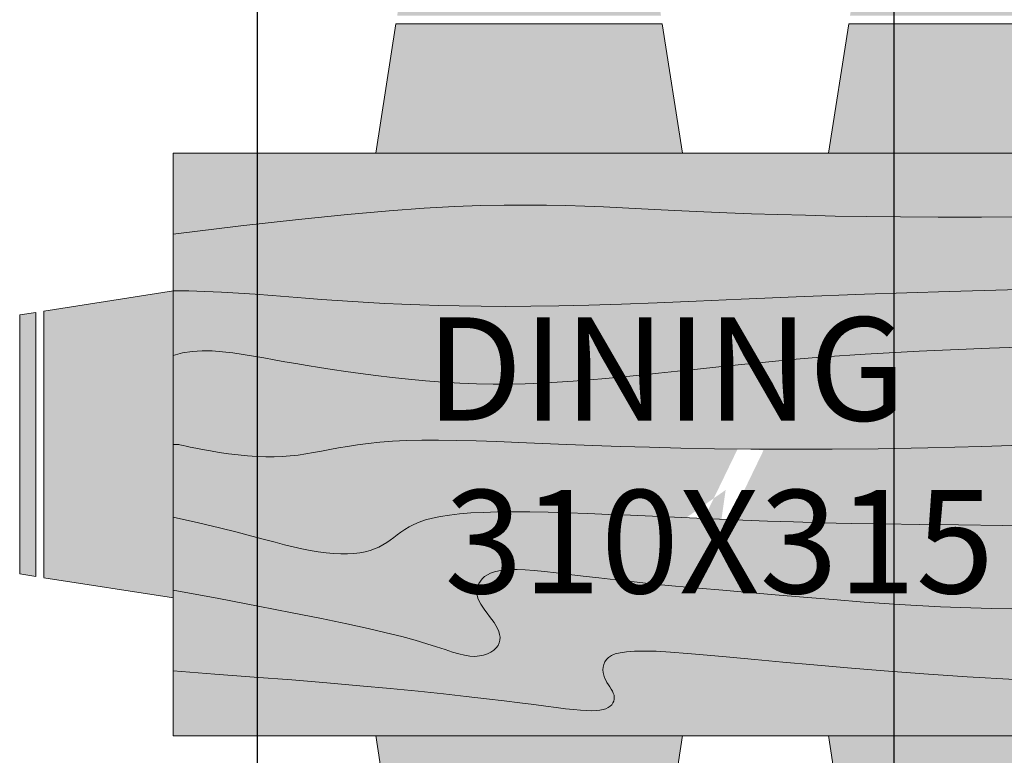
# Model space of a CAD drawing. Units: inches. Extents: x 192 to 1361, y -1362 to 367.
# Tile 16 of 23: x 498 to 662, y -337 to -214. Entities that reach past the tile are written whole.
import ezdxf

# ---------------------------------------------------------------- set-up
doc = ezdxf.new("R2010")
doc.units = ezdxf.units.IN
doc.header["$MEASUREMENT"] = 0
for name, color, linetype, lineweight in [('A-ANNO-DIMS', 2, 'Continuous', 18), ('A-AREA-IDEN', 7, 'Continuous', 18), ('furniture', 32, 'Continuous', 18)]:
    doc.layers.add(name, color=color, linetype=linetype, lineweight=lineweight)
doc.layers.add('A-FURN-PATT', color=254, linetype='Continuous', lineweight=13, true_color=0xfeeab9)
doc.styles.get("Standard").update_dxf_attribs({"font": 'arial.ttf'})
doc.dimstyles.get("Standard").update_dxf_attribs({"dimtxt": 0.18, "dimasz": 0.18, "dimexe": 0.18, "dimexo": 0.0625, "dimgap": 0.09, "dimtad": 0, "dimtih": 1, "dimtoh": 1, "dimzin": 0, "dimdsep": 46, "dimlunit": 3, "dimtxsty": 'Standard', "dimcen": 0.09, "dimadec": 0, "dimazin": 0, "dimtfac": 1, "dimtofl": 0, "dimtmove": 0, "dimatfit": 3, "dimfxl": 1, "dimtolj": 1, "dimtzin": 0, "dimarcsym": 0})

# ---------------------------------------------------------------- blocks, each defined once
blk = doc.blocks.new('Dining Set - 36 x 72 in.')
for p, q in [((-4.5152, 17.99762), (-5.7655, 25.99926)), ((5.7657, 26.00059), (4.5153, 17.99762)), ((23.4848, 17.99762), (22.2345, 25.99926)), ((36, 18), (-36, 18)), ((36, -18), (36, 18)), ((44.0006, 8.23428), (35.9976, 9.48474)), ((44, 8.23041), (44, -8.23915)), ((44.5, -8.15843), (44.5, 8.15338)), ((45.5, 8), (44.5005, 8.15617)), ((45.5, 8), (45.5, -8)), ((35.9976, -9.48476), (43.9993, -8.2345)), ((44.4997, -8.15631), (45.5, -8)), ((-36, -18), (36, -18)), ((-4.5152, -17.99762), (-5.7655, -25.99928)), ((5.7657, -26.0006), (4.5153, -17.99762)), ((23.4848, -17.99762), (22.2345, -25.99928)), ((-22.2304, -26), (-5.7608, -26)), ((5.7696, -26), (22.2392, -26))]:
    blk.add_line(p, q)
for points in [[(-16.0362, 14.53613), (-13.0957, 14.36718), (-10.4159, 14.18652), (-7.9583, 14), (-5.6904, 13.81315), (-3.6035, 13.63021), (-1.6954, 13.45508), (0.0365, 13.29166), (1.5945, 13.14388), (2.9811, 13.01562), (4.1988, 12.9108), (5.25, 12.83333), (6.1393, 12.78613), (6.8802, 12.76823), (7.4883, 12.77767), (7.9792, 12.8125), (8.3685, 12.87077), (8.6719, 12.95052), (8.9049, 13.0498), (9.0833, 13.16666), (9.2205, 13.29899), (9.3216, 13.44401), (9.3895, 13.59879), (9.4271, 13.76041), (9.4373, 13.92594), (9.4232, 14.09245), (9.3875, 14.257), (9.3333, 14.41666), (9.2638, 14.56917), (9.1836, 14.71484), (9.0975, 14.85465), (9.0104, 14.98958), (8.9272, 15.1206), (8.8529, 15.2487), (8.7922, 15.37483), (8.75, 15.5), (8.7305, 15.62467), (8.7344, 15.74739), (8.7617, 15.86621), (8.8125, 15.97916), (8.8867, 16.08431), (8.9844, 16.17968), (9.1055, 16.26334), (9.25, 16.33333), (9.4189, 16.38802), (9.6172, 16.42708), (9.8506, 16.45052), (10.125, 16.45833), (10.4463, 16.45052), (10.8203, 16.42708), (11.2529, 16.38802), (11.75, 16.33333), (12.3184, 16.26318), (12.9694, 16.17838), (13.7151, 16.07991), (14.5677, 15.96875), (15.5395, 15.84586), (16.6426, 15.71224), (17.8893, 15.56884), (19.2917, 15.41666), (20.859, 15.25667), (22.5879, 15.08984), (24.4721, 14.91715), (26.5052, 14.73958), (28.6809, 14.5581), (30.9929, 14.3737), (33.4347, 14.18733), (36, 14)], [(-18.4241, 10.19775), (-14.5677, 10.13541), (-11.4399, 10.03011), (-8.877, 9.89453), (-6.7154, 9.74137), (-4.7917, 9.58333), (-2.9698, 9.43082), (-1.2246, 9.28515), (0.4415, 9.14534), (2.026, 9.01041), (3.5266, 8.87939), (4.9408, 8.7513), (6.266, 8.62516), (7.5, 8.5), (8.6411, 8.37549), (9.6914, 8.2539), (10.6538, 8.13818), (11.5312, 8.03125), (12.3267, 7.93603), (13.043, 7.85547), (13.6831, 7.79248), (14.25, 7.75), (14.7471, 7.7303), (15.1797, 7.73307), (15.5537, 7.75732), (15.875, 7.80208), (16.1494, 7.86637), (16.3828, 7.94922), (16.5811, 8.04964), (16.75, 8.16666), (16.8944, 8.29915), (17.0143, 8.44531), (17.1089, 8.60319), (17.1771, 8.77083), (17.218, 8.94629), (17.2305, 9.1276), (17.2137, 9.31282), (17.1667, 9.5), (17.0895, 9.6875), (16.987, 9.875), (16.8649, 10.0625), (16.7292, 10.25), (16.5856, 10.4375), (16.4401, 10.625), (16.2985, 10.8125), (16.1667, 11), (16.05, 11.18733), (15.9518, 11.3737), (15.8752, 11.5581), (15.8229, 11.73958), (15.798, 11.91715), (15.8034, 12.08984), (15.842, 12.25667), (15.9167, 12.41666), (16.0295, 12.56836), (16.1784, 12.70833), (16.3605, 12.83268), (16.5729, 12.9375), (16.8127, 13.01888), (17.0768, 13.07291), (17.3625, 13.0957), (17.6667, 13.08333), (17.9894, 13.03312), (18.3418, 12.94726), (18.7382, 12.82918), (19.1927, 12.68229), (19.7195, 12.51001), (20.3327, 12.31575), (21.0465, 12.10294), (21.875, 11.875), (22.8357, 11.63354), (23.959, 11.37304), (25.2786, 11.08618), (26.8282, 10.76562), (28.6414, 10.40405), (30.752, 9.99414), (33.1936, 9.52856), (36, 9)], [(-18.4271, 5.05208), (-15.3009, 5.00602), (-12.5508, 4.97265), (-10.1112, 4.94515), (-7.9167, 4.91666), (-5.909, 4.88167), (-4.0586, 4.83984), (-2.3429, 4.79215), (-0.7396, 4.73958), (0.7739, 4.6831), (2.22, 4.6237), (3.6213, 4.56233), (5, 4.5), (6.373, 4.43782), (7.7344, 4.3776), (9.0723, 4.32129), (10.375, 4.27083), (11.6309, 4.22819), (12.8281, 4.19531), (13.9551, 4.17415), (15, 4.16666), (15.954, 4.17448), (16.819, 4.19791), (17.6001, 4.23698), (18.3021, 4.29166), (18.9299, 4.36198), (19.4883, 4.44791), (19.9823, 4.54948), (20.4167, 4.66666), (20.7969, 4.79899), (21.1302, 4.94401), (21.4245, 5.09879), (21.6875, 5.26041), (21.9271, 5.42594), (22.1511, 5.59245), (22.3672, 5.757), (22.5834, 5.91666), (22.8065, 6.06868), (23.0404, 6.21093), (23.2879, 6.34147), (23.5521, 6.45833), (23.8358, 6.55957), (24.142, 6.64323), (24.4735, 6.70735), (24.8334, 6.75), (25.2235, 6.76969), (25.642, 6.76692), (26.0858, 6.74267), (26.5521, 6.69791), (27.0379, 6.63362), (27.5404, 6.55078), (28.0565, 6.45036), (28.5834, 6.33333), (29.1242, 6.19987), (29.7071, 6.04687), (30.3661, 5.87044), (31.1354, 5.66666), (32.0493, 5.43164), (33.142, 5.16146), (34.4475, 4.85221), (36, 4.5)], [(-17.6563, 0.00521), (-14.0005, 0.12833), (-10.6523, 0.21289), (-7.5796, 0.26522), (-4.75, 0.29166), (-2.134, 0.29793), (0.2878, 0.28711), (2.5317, 0.26163), (4.6146, 0.22396), (6.5529, 0.17651), (8.3633, 0.12174), (10.0623, 0.06209), (11.6667, 0), (13.1899, -0.06201), (14.6341, -0.1211), (15.9982, -0.17432), (17.2813, -0.21875), (18.4823, -0.25147), (19.6003, -0.26953), (20.6343, -0.27002), (21.5834, -0.25), (22.4481, -0.20768), (23.2357, -0.14584), (23.9549, -0.06836), (24.6146, 0.02083), (25.2235, 0.11784), (25.7904, 0.21875), (26.3241, 0.31966), (26.8334, 0.41666), (27.3265, 0.50618), (27.8099, 0.58593), (28.2894, 0.65397), (28.7709, 0.70833), (29.2601, 0.74707), (29.763, 0.76823), (30.2855, 0.76985), (30.8334, 0.75), (31.4088, 0.70784), (31.9994, 0.64713), (32.589, 0.57275), (33.1615, 0.48958), (33.7008, 0.4025), (34.1908, 0.3164), (34.6153, 0.23616), (34.9584, 0.16666), (35.2099, 0.11165), (35.3848, 0.07031), (35.504, 0.04069), (35.5886, 0.02083), (35.6594, 0.00879), (35.7377, 0.0026), (35.8442, 0.00032), (36, 0)], [(-20.084, -6.1263), (-14.469, -5.9419), (-10.1094, -5.76042), (-6.7752, -5.58285), (-4.2363, -5.41016), (-2.2629, -5.24333), (-0.625, -5.08334), (0.8708, -4.93099), (2.2715, -4.78646), (3.5872, -4.64974), (4.8281, -4.52084), (6.0046, -4.39974), (7.127, -4.28646), (8.2053, -4.18099), (9.25, -4.08334), (10.2705, -3.99382), (11.2734, -3.91407), (12.2647, -3.84603), (13.25, -3.79167), (14.2354, -3.75293), (15.2266, -3.73177), (16.2295, -3.73015), (17.25, -3.75), (18.2912, -3.79248), (19.3451, -3.85547), (20.4009, -3.93604), (21.4479, -4.03125), (22.4754, -4.13819), (23.4727, -4.25391), (24.4289, -4.37549), (25.3334, -4.5), (26.1785, -4.62492), (26.9694, -4.74935), (27.7145, -4.87281), (28.4219, -4.99479), (29.1, -5.11483), (29.7572, -5.23242), (30.4016, -5.34709), (31.0417, -5.45834), (31.6837, -5.56437), (32.3262, -5.65821), (32.9658, -5.73153), (33.599, -5.77604), (34.2224, -5.78345), (34.8327, -5.74545), (35.4264, -5.65373), (36, -5.5)], [(-18.4675, -9.62891), (-11.9839, -9.45069), (-6.7396, -9.28125), (-2.5226, -9.12354), (0.8789, -8.98047), (3.6769, -8.85498), (6.0833, -8.75), (8.2767, -8.66765), (10.3021, -8.60677), (12.1712, -8.56543), (13.8958, -8.54167), (15.4876, -8.53353), (16.9583, -8.53907), (18.3197, -8.55632), (19.5834, -8.58334), (20.7616, -8.61841), (21.8685, -8.66081), (22.9188, -8.71004), (23.9271, -8.76563), (24.9081, -8.82707), (25.8763, -8.89388), (26.8465, -8.96558), (27.8334, -9.04167), (28.8474, -9.12118), (29.8828, -9.20117), (30.93, -9.27824), (31.9792, -9.34896), (33.0205, -9.40991), (34.0443, -9.45768), (35.0407, -9.48885), (36, -9.5)], [(-17.0781, -14.07292), (-13.97, -14.04671), (-11.3027, -14.04297), (-8.9724, -14.05681), (-6.875, -14.08334), (-4.9224, -14.11833), (-3.0905, -14.16016), (-1.3709, -14.20785), (0.2448, -14.26042), (1.7647, -14.3169), (3.1973, -14.3763), (4.5507, -14.43767), (5.8333, -14.5), (7.0554, -14.5621), (8.235, -14.62175), (9.3922, -14.67652), (10.5469, -14.72396), (11.7192, -14.76164), (12.929, -14.78711), (14.1965, -14.79794), (15.5417, -14.79167), (16.9933, -14.76424), (18.6152, -14.70508), (20.4804, -14.60197), (22.6615, -14.44271), (25.2312, -14.21509), (28.2624, -13.9069), (31.8277, -13.50594), (36, -13)]]:
    blk.add_lwpolyline(points)
blk = doc.blocks.new('dining area')
at = {"layer": 'furniture', "xscale": 0.6659924291999282, "yscale": 0.6659924291999282, "zscale": 0.6659924291999282, "rotation": 90}
blk.add_blockref('Dining Set - 36 x 72 in.', (-0.439, 20.507), dxfattribs=at)
blk = doc.blocks.new('*D70')
at = {"layer": 'A-ANNO-DIMS', "color": 0, "lineweight": -2, "transparency": 16777216}
for p, q in [((537.57, -441.84), (537.57, 367.39)), ((537.75, 367.21), (590.28, 367.21)), ((643.71, 367.21), (591.19, 367.21)), ((643.89, -441.84), (643.89, 367.39))]:
    blk.add_line(p, q, dxfattribs=at)
at = {"layer": 'A-ANNO-DIMS', "color": 0, "transparency": 16777216}
for points in [[(537.75, 367.24), (537.75, 367.18), (537.57, 367.21)], [(643.71, 367.24), (643.71, 367.18), (643.89, 367.21)]]:
    blk.add_solid(points, dxfattribs=at)
at = {"layer": 'Defpoints', "color": 0, "transparency": 16777216}
for p in [(643.89, 367.21), (537.57, -441.9), (643.89, -441.9)]:
    blk.add_point(p, dxfattribs=at)
at = {"layer": 'A-ANNO-DIMS', "color": 0, "transparency": 16777216, "insert": (590.73, 367.21), "char_height": 0.18, "attachment_point": 5}
blk.add_mtext('\\A1;106.32', dxfattribs=at)

msp = doc.modelspace()

# ---------------------------------------------------------------- hatches: boundary and pattern name
at = {"layer": 'A-FURN-PATT'}
h = msp.add_hatch(color=256, dxfattribs=at)
h.dxf.hatch_style = 1
h.paths.add_polyline_path([(605.1742, -214.7906), (560.6934, -214.7906), (557.3171, -236.398), (608.5502, -236.398)])
h.paths.add_polyline_path([(604.5412, -210.7392), (561.3264, -210.7392), (560.9044, -213.4402), (604.9632, -213.4402)])
h.paths.add_polyline_path([(680.8, -214.7906), (636.3191, -214.7906), (632.9429, -236.398), (684.176, -236.398)])
h.paths.add_polyline_path([(680.1669, -210.7392), (636.9522, -210.7392), (636.5302, -213.4402), (680.589, -213.4402)])
h.paths.add_polyline_path([(523.5135, -259.398), (501.9062, -262.7741), (501.9062, -307.2549), (523.5135, -310.6311)])
h.paths.add_polyline_path([(500.5557, -262.9851), (497.8548, -263.4072), (497.8548, -306.6219), (500.5557, -307.0439)])
h.paths.add_polyline_path([(608.5502, -333.6311), (557.3171, -333.6311), (560.6934, -355.2385), (605.1742, -355.2385)])
h.paths.add_polyline_path([(604.9632, -356.5889), (560.9044, -356.5889), (561.3264, -359.2899), (604.5412, -359.2899)])
h.paths.add_polyline_path([(680.589, -356.5889), (636.5302, -356.5889), (636.9522, -359.2899), (680.1669, -359.2899)])
h.paths.add_polyline_path([(684.176, -333.6311), (632.9429, -333.6311), (636.3191, -355.2385), (680.8, -355.2385)])
h.paths.add_polyline_path([(739.5872, -262.7741), (717.9798, -259.398), (717.9798, -310.6311), (739.5872, -307.2549)])
h.paths.add_polyline_path([(743.6386, -263.4072), (740.9376, -262.9851), (740.9376, -307.0439), (743.6386, -306.6219)])
h = msp.add_hatch(color=256, dxfattribs=at)
h.dxf.hatch_style = 1
h.paths.add_polyline_path([(717.9798, -236.398), (523.5135, -236.398), (523.5135, -249.9026), (534.7826, -248.5361), (544.4122, -247.4531), (552.5992, -246.6207), (559.5398, -246.0059), (565.4307, -245.5758), (570.4685, -245.2973), (574.8491, -245.1375), (578.7698, -245.0634), (582.4031, -245.0465), (585.8265, -245.0757), (589.094, -245.1445), (592.2603, -245.2463), (595.3791, -245.3744), (598.5046, -245.5224), (601.6906, -245.6835), (604.9914, -245.8512), (608.4556, -246.0195), (612.111, -246.1853), (615.9804, -246.3457), (620.0855, -246.4983), (624.4494, -246.6403), (629.0939, -246.7691), (634.0417, -246.8821), (639.3155, -246.9766), (644.9804, -247.0482), (651.2744, -247.0856), (658.4785, -247.0755), (666.8733, -247.0047), (676.74, -246.8601), (688.3594, -246.6284), (702.0122, -246.2965), (717.9798, -245.8512)])
h.paths.add_polyline_path([(717.9798, -245.8512), (702.0122, -246.2965), (688.3594, -246.6284), (676.74, -246.8601), (666.8733, -247.0047), (658.4785, -247.0755), (651.2744, -247.0856), (644.9804, -247.0482), (639.3155, -246.9766), (634.0417, -246.8821), (629.0939, -246.7691), (624.4494, -246.6403), (620.0855, -246.4983), (615.9804, -246.3457), (612.111, -246.1853), (608.4556, -246.0195), (604.9914, -245.8512), (601.6906, -245.6835), (598.5046, -245.5224), (595.3791, -245.3744), (592.2603, -245.2463), (589.094, -245.1445), (585.8265, -245.0757), (582.4031, -245.0465), (578.7698, -245.0634), (574.8491, -245.1375), (570.4685, -245.2973), (565.4307, -245.5758), (559.5398, -246.0059), (552.5992, -246.6207), (544.4122, -247.4531), (534.7826, -248.5361), (523.5135, -249.9026), (523.5135, -259.3558), (526.1045, -259.3859), (528.7957, -259.4701), (531.5609, -259.5991), (534.3734, -259.7638), (537.2072, -259.9548), (540.0356, -260.1629), (542.8321, -260.379), (545.5709, -260.5937), (548.2364, -260.7992), (550.8568, -260.9929), (553.4719, -261.1733), (556.1215, -261.3393), (558.8448, -261.4894), (561.6816, -261.6224), (564.6712, -261.7369), (567.8535, -261.8316), (571.2666, -261.9046), (574.9437, -261.9512), (578.9159, -261.9662), (583.2152, -261.9442), (587.8732, -261.88), (592.9215, -261.7683), (598.392, -261.6039), (604.3162, -261.3815), (610.8157, -261.098), (618.3728, -260.759), (627.56, -260.3726), (638.9498, -259.9466), (653.1142, -259.489), (670.6259, -259.0076), (692.0569, -258.5104), (717.9798, -258.0053)])
h.paths.add_polyline_path([(602.4999, -265.0738), (602.0375, -261.467), (598.392, -261.6039), (592.9215, -261.7683), (587.8732, -261.88), (583.2152, -261.9442), (578.9159, -261.9662), (574.9437, -261.9512), (571.2666, -261.9046), (567.8535, -261.8316), (564.6712, -261.7369), (561.6816, -261.6224), (558.8448, -261.4894), (556.1215, -261.3393), (553.4719, -261.1733), (550.8568, -260.9929), (548.2364, -260.7992), (545.5709, -260.5937), (542.8321, -260.379), (540.0356, -260.1629), (537.2072, -259.9548), (534.3734, -259.7638), (531.5609, -259.5991), (528.7957, -259.4701), (526.1045, -259.3859), (523.7648, -259.3587), (523.5135, -259.398), (523.5135, -270.1595), (525.0628, -269.7443), (526.6663, -269.4965), (528.3147, -269.3939), (529.9984, -269.4139), (531.7087, -269.5341), (533.4362, -269.7322), (535.1715, -269.9856), (536.9055, -270.272), (538.6344, -270.5725), (540.3748, -270.8822), (542.1499, -271.1998), (543.9814, -271.524), (545.892, -271.8535), (547.9045, -272.1869), (550.0406, -272.523), (552.3232, -272.8604), (554.7662, -273.1967), (557.3488, -273.5251), (560.0424, -273.8376), (562.8176, -274.1265), (565.6455, -274.3836), (568.4971, -274.6012), (571.3436, -274.7714), (574.1558, -274.8861), (576.9121, -274.9397), (579.6208, -274.9353), (582.298, -274.8782), (584.9595, -274.7735), (587.6207, -274.6267), (590.2981, -274.443), (593.0069, -274.2276), (595.7632, -273.9858), (598.5848, -273.722), (601.4972, -273.4372), (604.5287, -273.1312), (607.7064, -272.8041), (611.0579, -272.456), (611.8813, -272.3704)])
h.paths.add_polyline_path([(613.2364, -275.1581), (604.0875, -273.1757), (601.4972, -273.4372), (598.5848, -273.722), (595.7632, -273.9858), (593.0069, -274.2276), (590.2981, -274.443), (587.6207, -274.6267), (584.9595, -274.7735), (582.298, -274.8782), (579.6208, -274.9353), (576.9121, -274.9397), (574.1558, -274.8861), (571.3436, -274.7714), (568.4971, -274.6012), (565.6455, -274.3836), (562.8176, -274.1265), (560.0424, -273.8376), (557.3488, -273.5251), (554.7662, -273.1967), (552.3232, -272.8604), (550.0406, -272.523), (547.9045, -272.1869), (545.892, -271.8535), (543.9814, -271.524), (542.1499, -271.1998), (540.3748, -270.8822), (538.6344, -270.5725), (536.9055, -270.272), (535.1715, -269.9856), (533.4362, -269.7322), (531.7087, -269.5341), (529.9984, -269.4139), (528.3147, -269.3939), (526.6663, -269.4965), (525.0628, -269.7443), (523.5135, -270.1595), (523.5135, -285.0145), (524.3927, -285.0164), (524.8532, -285.1244), (525.1751, -285.2045), (525.6475, -285.3161), (526.3268, -285.4647), (527.2535, -285.6524), (528.4, -285.8691), (529.7235, -286.1017), (531.1801, -286.3369), (532.7264, -286.5615), (534.3188, -286.7624), (535.914, -286.9264), (537.4681, -287.0402), (538.9479, -287.0939), (540.3592, -287.0895), (541.7175, -287.0323), (543.0388, -286.9277), (544.3393, -286.7809), (545.6343, -286.5971), (546.94, -286.3817), (548.2718, -286.1399), (549.6474, -285.8779), (551.0889, -285.6054), (552.62, -285.3328), (554.2646, -285.0708), (556.0464, -284.8299), (557.9889, -284.6206), (560.1161, -284.4536), (562.4516, -284.3393), (565.0151, -284.2852), (567.8078, -284.2866), (570.8275, -284.3353), (574.0713, -284.4237), (577.5368, -284.5437), (581.2211, -284.6875), (585.1218, -284.8471), (589.2358, -285.0145), (593.5692, -285.1822), (598.1581, -285.3434), (603.0478, -285.4913), (608.283, -285.6194), (613.9088, -285.7212), (616.4226, -285.7497), (616.7471, -285.69)], flags=16)
h.paths.add_polyline_path([(717.9798, -258.0053), (692.0569, -258.5104), (670.6259, -259.0076), (653.1142, -259.489), (638.9498, -259.9466), (627.56, -260.3726), (618.3728, -260.759), (610.8157, -261.098), (604.3162, -261.3815), (602.0375, -261.467), (602.4999, -265.0738), (611.8813, -272.3704), (614.6115, -272.0867), (618.3947, -271.6963), (622.4348, -271.2849), (627.3208, -270.8076), (627.3197, -270.8137), (632.1886, -270.4021), (639.046, -269.9357), (648.0514, -269.4561), (659.8263, -268.9659), (674.992, -268.4679), (694.1693, -267.9645), (717.9798, -267.4586)])
h.paths.add_polyline_path([(717.9798, -267.4586), (694.1693, -267.9645), (674.992, -268.4679), (659.8263, -268.9659), (648.0514, -269.4561), (639.046, -269.9357), (637.7073, -270.0268), (634.981, -274.8872), (634.93, -274.8716), (627.474, -277.1084), (618.2223, -284.5098), (623.8182, -285.8072), (626.5104, -285.8192), (633.576, -285.8023), (641.2186, -285.7309), (649.5177, -285.5895), (658.5609, -285.3612), (668.4349, -285.0286), (679.2267, -284.5747), (691.0233, -283.9824), (703.9121, -283.2344), (717.9798, -282.3136)])
h.paths.add_polyline_path([(717.9798, -282.3136), (703.9121, -283.2344), (691.0233, -283.9824), (679.2267, -284.5747), (668.4349, -285.0286), (658.5609, -285.3612), (649.5177, -285.5895), (641.2186, -285.7309), (633.576, -285.8023), (626.5104, -285.8192), (619.9694, -285.79), (616.8026, -285.7541), (623.8185, -293.8493), (623.9185, -293.8319), (623.9419, -293.9917), (626.0437, -296.4169), (628.742, -298.0041), (631.7086, -298.0866), (636.7064, -298.1996), (642.1291, -298.2941), (648.0562, -298.371), (654.6454, -298.4453), (662.0732, -298.5354), (670.5168, -298.6598), (680.1523, -298.837), (691.157, -299.0853), (703.7073, -299.4234), (717.9798, -299.8696)])
h.paths.add_polyline_path([(717.9798, -299.8696), (703.7073, -299.4234), (691.157, -299.0853), (680.1523, -298.837), (670.5168, -298.6598), (662.0732, -298.5354), (654.6454, -298.4453), (648.0562, -298.371), (642.1291, -298.2941), (636.7064, -298.1996), (631.7086, -298.0866), (628.742, -298.0041), (626.0437, -296.4169), (623.9419, -293.9917), (616.8026, -285.7541), (616.738, -285.7533), (614.6017, -300.7077), (613.756, -301.5533), (614.1357, -309.2515), (615.2746, -309.351), (619.5542, -309.7154), (624.0542, -310.093), (628.7679, -310.4864), (633.6887, -310.8984), (638.8844, -311.3252), (644.7227, -311.7389), (651.6449, -312.1051), (660.0929, -312.3895), (670.5087, -312.5579), (683.3338, -312.5759), (699.0102, -312.4093), (717.9798, -312.0238)], flags=17)
h.paths.add_polyline_path([(615.758, -292.6135), (616.7471, -285.69), (613.2364, -275.1581), (604.0875, -273.1757), (601.4972, -273.4372), (598.5848, -273.722), (595.7632, -273.9858), (593.0069, -274.2276), (590.2981, -274.443), (587.6207, -274.6267), (584.9595, -274.7735), (582.298, -274.8782), (579.6208, -274.9353), (576.9121, -274.9397), (574.1558, -274.8861), (571.3436, -274.7714), (568.4971, -274.6012), (565.6455, -274.3836), (562.8176, -274.1265), (560.0424, -273.8376), (557.3488, -273.5251), (554.7662, -273.1967), (552.3232, -272.8604), (550.0406, -272.523), (547.9045, -272.1869), (545.892, -271.8535), (543.9814, -271.524), (542.1499, -271.1998), (540.3748, -270.8822), (538.6344, -270.5725), (536.9055, -270.272), (535.1715, -269.9856), (533.4362, -269.7322), (531.7087, -269.5341), (529.9984, -269.4139), (528.3147, -269.3939), (526.6663, -269.4965), (525.0628, -269.7443), (523.5135, -270.1595), (523.5135, -285.0145), (524.3927, -285.0164), (524.8532, -285.1244), (525.1751, -285.2045), (525.9724, -285.3929), (526.3268, -285.4647), (525.4551, -285.274), (524.8532, -285.1244), (524.3927, -285.0164), (523.5135, -285.0145), (523.5135, -297.1687), (527.7067, -298.12), (531.2328, -298.9552), (534.1841, -299.685), (536.6524, -300.3197), (538.7303, -300.8701), (540.5102, -301.3467), (542.0845, -301.7599), (543.5452, -302.1204), (544.9683, -302.4365), (546.3622, -302.7077), (547.7195, -302.9314), (549.0316, -303.1051), (550.291, -303.226), (551.4897, -303.2915), (552.62, -303.2989), (553.6736, -303.2458), (554.6457, -303.1306), (555.5411, -302.9574), (556.3681, -302.7314), (557.1343, -302.458), (557.8479, -302.1424), (558.5164, -301.7898), (559.1481, -301.4056), (559.7507, -300.995), (560.3346, -300.5637), (561.3682, -299.7768), (562.1705, -299.2225), (562.8808, -298.786), (563.6757, -298.3679), (564.5759, -297.9762), (565.6028, -297.6188), (566.7761, -297.3023), (568.1103, -297.028), (569.6185, -296.7959), (571.3142, -296.606), (573.2102, -296.4583), (575.3199, -296.3528), (577.6562, -296.2895), (580.2329, -296.2684), (583.0551, -296.2886), (586.099, -296.3457), (589.3325, -296.4346), (592.7246, -296.5497), (596.2431, -296.686), (599.8567, -296.8381), (603.5337, -297.0007), (607.2421, -297.1687), (609.1466, -297.2548)])
h.paths.add_polyline_path([(614.6017, -300.7077), (615.758, -292.6135), (609.1466, -297.2548), (607.2421, -297.1687), (603.5337, -297.0007), (599.8567, -296.8381), (596.2431, -296.686), (592.7246, -296.5497), (589.3325, -296.4346), (586.099, -296.3457), (583.0551, -296.2886), (580.2329, -296.2684), (577.6562, -296.2895), (575.3199, -296.3528), (573.2102, -296.4583), (571.3142, -296.606), (569.6185, -296.7959), (568.1103, -297.028), (566.7761, -297.3023), (565.6028, -297.6188), (564.5759, -297.9762), (563.6757, -298.3679), (562.8808, -298.786), (562.1705, -299.2225), (561.3682, -299.7768), (559.9183, -300.8808), (558.8169, -301.6313), (557.8479, -302.1424), (557.1343, -302.458), (556.3681, -302.7314), (555.5411, -302.9574), (554.6457, -303.1306), (553.6736, -303.2458), (552.62, -303.2989), (551.4897, -303.2915), (550.291, -303.226), (549.0316, -303.1051), (547.7195, -302.9314), (546.3622, -302.7077), (544.9683, -302.4365), (543.5452, -302.1204), (542.0845, -301.7599), (540.5102, -301.3467), (538.7303, -300.8701), (536.6524, -300.3197), (534.1841, -299.685), (531.2328, -298.9552), (527.7067, -298.12), (523.5135, -297.1687), (523.5135, -309.3228), (531.0934, -310.7504), (537.688, -312.0079), (543.3885, -313.1151), (548.2858, -314.0916), (552.4712, -314.9574), (556.0353, -315.7322), (559.0693, -316.4358), (561.664, -317.088), (563.9018, -317.7036), (565.8297, -318.2784), (567.4859, -318.8031), (568.9087, -319.2684), (570.1363, -319.6651), (571.2069, -319.9841), (572.1587, -320.216), (573.0303, -320.3516), (573.8519, -320.385), (574.6236, -320.3234), (575.3369, -320.1775), (575.9846, -319.9577), (576.5583, -319.6746), (577.0501, -319.3387), (577.4523, -318.9607), (577.7569, -318.551), (577.9587, -318.1188), (578.0629, -317.6682), (578.0775, -317.2018), (578.0103, -316.7222), (577.869, -316.2321), (577.6621, -315.734), (577.3969, -315.2306), (577.0817, -314.7247), (576.7257, -314.2183), (576.3433, -313.7118), (575.6335, -312.7972), (574.9795, -311.8936), (574.4388, -310.9045), (574.1912, -309.9182), (574.259, -308.9341), (574.6297, -308.023), (575.2828, -307.2269), (576.2025, -306.5897), (577.1284, -306.261), (577.8696, -306.0873), (578.7374, -305.9665), (579.7475, -305.901), (580.9159, -305.8935), (582.2586, -305.9467), (583.7897, -306.0614), (585.5186, -306.2315), (587.4532, -306.4491), (589.6018, -306.7063), (591.9716, -306.9951), (594.571, -307.3077), (597.4078, -307.6361), (600.4898, -307.9724), (603.8227, -308.3104), (606.7229, -308.5865)], flags=0)
h.paths.add_polyline_path([(613.2364, -275.1581), (604.0875, -273.1757), (601.4972, -273.4372), (598.5848, -273.722), (595.7632, -273.9858), (593.0069, -274.2276), (590.2981, -274.443), (587.6207, -274.6267), (584.9595, -274.7735), (582.298, -274.8782), (579.6208, -274.9353), (576.9121, -274.9397), (574.1558, -274.8861), (571.3436, -274.7714), (568.4971, -274.6012), (565.6455, -274.3836), (562.8176, -274.1265), (560.0424, -273.8376), (557.3488, -273.5251), (554.7662, -273.1967), (552.3232, -272.8604), (550.0406, -272.523), (547.9045, -272.1869), (545.892, -271.8535), (543.9814, -271.524), (542.1499, -271.1998), (540.3748, -270.8822), (538.6344, -270.5725), (536.9055, -270.272), (535.1715, -269.9856), (533.4362, -269.7322), (531.7087, -269.5341), (529.9984, -269.4139), (528.3147, -269.3939), (526.6663, -269.4965), (525.0628, -269.7443), (523.5135, -270.1595), (523.5135, -285.0145), (523.9343, -285.0154), (524.3927, -285.0164), (524.8532, -285.1244), (525.1751, -285.2045), (525.6475, -285.3161), (526.3268, -285.4647), (527.2535, -285.6524), (528.4, -285.8691), (529.7235, -286.1017), (531.1801, -286.3369), (532.7264, -286.5615), (534.3188, -286.7624), (535.914, -286.9264), (537.4681, -287.0402), (538.9479, -287.0939), (540.3592, -287.0895), (541.7175, -287.0323), (543.0388, -286.9277), (544.3393, -286.7809), (545.6343, -286.5971), (546.94, -286.3817), (548.2718, -286.1399), (549.6474, -285.8779), (551.0889, -285.6054), (552.62, -285.3328), (554.2646, -285.0708), (556.0464, -284.8299), (557.9889, -284.6206), (560.1161, -284.4536), (562.4516, -284.3393), (565.0151, -284.2852), (567.8078, -284.2866), (570.8275, -284.3353), (574.0713, -284.4237), (577.5368, -284.5437), (581.2211, -284.6875), (585.1218, -284.8471), (589.2358, -285.0145), (593.5692, -285.1822), (598.1581, -285.3434), (603.0478, -285.4913), (608.283, -285.6194), (613.9088, -285.7212), (616.4226, -285.7497), (616.7471, -285.69)], flags=17)
h.paths.add_polyline_path([(575.9846, -319.9577), (576.5583, -319.6746), (577.0501, -319.3387), (577.4523, -318.9607), (577.7569, -318.551), (577.9587, -318.1188), (578.0629, -317.6682), (578.0775, -317.2018), (578.0103, -316.7222), (577.869, -316.2321), (577.6621, -315.734), (577.3969, -315.2306), (577.0817, -314.7247), (576.7257, -314.2183), (576.3433, -313.7118), (575.3608, -312.4458), (575.1959, -312.1926), (574.9795, -311.8936), (574.4388, -310.9045), (574.1912, -309.9182), (574.259, -308.9341), (574.6297, -308.023), (575.2828, -307.2269), (576.2025, -306.5897), (577.1284, -306.261), (577.8696, -306.0873), (578.7374, -305.9665), (579.7475, -305.901), (580.9159, -305.8935), (582.2586, -305.9467), (583.7897, -306.0614), (585.5186, -306.2315), (587.4532, -306.4491), (589.6018, -306.7063), (591.9716, -306.9951), (594.571, -307.3077), (597.4078, -307.6361), (600.4898, -307.9724), (603.8227, -308.3104), (606.7229, -308.5865), (614.6017, -300.7077), (615.758, -292.6135), (609.1466, -297.2548), (607.2421, -297.1687), (603.5337, -297.0007), (599.8567, -296.8381), (596.2431, -296.686), (592.7246, -296.5497), (589.3325, -296.4346), (586.099, -296.3457), (583.0551, -296.2886), (580.2329, -296.2684), (577.6562, -296.2895), (575.3199, -296.3528), (573.2102, -296.4583), (571.3142, -296.606), (569.6185, -296.7959), (568.1103, -297.028), (566.7761, -297.3023), (565.6028, -297.6188), (564.5759, -297.9762), (563.6757, -298.3679), (562.8808, -298.786), (562.1705, -299.2225), (561.3682, -299.7768), (559.9183, -300.8808), (558.8169, -301.6313), (557.8479, -302.1424), (557.1343, -302.458), (556.3681, -302.7314), (555.5411, -302.9574), (554.6457, -303.1306), (553.6736, -303.2458), (552.62, -303.2989), (551.4897, -303.2915), (550.291, -303.226), (549.0316, -303.1051), (547.7195, -302.9314), (546.3622, -302.7077), (544.9683, -302.4365), (543.5452, -302.1204), (542.0845, -301.7599), (540.5102, -301.3467), (538.7303, -300.8701), (536.6524, -300.3197), (534.1841, -299.685), (531.2328, -298.9552), (527.7067, -298.12), (523.5135, -297.1687), (523.5135, -309.3228), (531.0934, -310.7504), (537.688, -312.0079), (543.3885, -313.1151), (548.2858, -314.0916), (552.4712, -314.9574), (556.0353, -315.7322), (559.0693, -316.4358), (561.664, -317.088), (563.9018, -317.7036), (565.8297, -318.2784), (567.4859, -318.8031), (568.9087, -319.2684), (570.1363, -319.6651), (571.2069, -319.9841), (572.1587, -320.216), (573.0303, -320.3516), (573.8519, -320.385), (574.6236, -320.3234), (575.3369, -320.1775)], flags=17)
h.paths.add_polyline_path([(606.7229, -308.5865), (603.8227, -308.3104), (600.4898, -307.9724), (597.4078, -307.6361), (594.571, -307.3077), (591.9716, -306.9951), (589.6018, -306.7063), (587.4532, -306.4491), (585.5186, -306.2315), (583.7897, -306.0614), (582.2586, -305.9467), (580.9159, -305.8935), (579.7475, -305.901), (578.7374, -305.9665), (577.8696, -306.0873), (577.1284, -306.261), (576.498, -306.4848), (575.9624, -306.756), (575.5063, -307.072), (575.1162, -307.4299), (574.7924, -307.8247), (574.5369, -308.2511), (574.3527, -308.7039), (574.2422, -309.1778), (574.2085, -309.6675), (574.2538, -310.1677), (574.3808, -310.6733), (574.5893, -311.1797), (574.8661, -311.6861), (575.1959, -312.1926), (575.5624, -312.699), (575.9503, -313.2054), (576.6244, -314.0741), (577.2758, -315.0008), (577.802, -315.9994), (578.0845, -316.9797), (578.0553, -317.9119), (577.6543, -318.7708), (576.8415, -319.5348), (575.6824, -320.1068), (574.6236, -320.3234), (573.8519, -320.385), (573.0303, -320.3516), (572.1587, -320.216), (571.2069, -319.9841), (570.1363, -319.6651), (568.9087, -319.2684), (567.4859, -318.8031), (565.8297, -318.2784), (563.9018, -317.7036), (561.664, -317.088), (559.0693, -316.4358), (556.0353, -315.7322), (552.4712, -314.9574), (548.2858, -314.0916), (543.3885, -313.1151), (537.688, -312.0079), (531.0934, -310.7504), (523.5135, -309.3228), (523.5135, -322.8274), (530.4422, -323.3334), (537.0373, -323.8368), (543.2818, -324.3348), (549.1582, -324.825), (554.6495, -325.3046), (559.7386, -325.771), (564.4082, -326.2216), (568.6413, -326.6537), (572.4291, -327.0647), (575.7963, -327.4521), (578.7757, -327.813), (581.4005, -328.1449), (583.7033, -328.4451), (585.7174, -328.7111), (587.4757, -328.9401), (589.0109, -329.1296), (590.3535, -329.2773), (591.5219, -329.3828), (592.5321, -329.4461), (593.3999, -329.4672), (594.141, -329.4461), (594.7714, -329.3828), (595.307, -329.2773), (595.7632, -329.1296), (596.1534, -328.9405), (596.4805, -328.7146), (596.7444, -328.457), (596.9448, -328.173), (597.082, -327.8679), (597.1558, -327.547), (597.1663, -327.2155), (597.1136, -326.8788), (596.9996, -326.5407), (596.8357, -326.2001), (596.635, -325.8541), (596.4103, -325.5002), (595.8425, -324.6206), (595.4373, -323.7315), (595.2441, -322.841), (595.2995, -321.9418), (595.6674, -321.1033), (596.4183, -320.379), (597.3246, -319.9929), (598.144, -319.7775), (599.1955, -319.6201), (600.5214, -319.526), (602.1638, -319.5005), (604.1649, -319.5489), (606.5668, -319.6764), (609.4061, -319.8856), (612.695, -320.1687), (616.4401, -320.5151), (620.6481, -320.9143), (625.3258, -321.3557), (630.4794, -321.8287), (636.116, -322.3228), (642.2414, -322.8274), (648.8792, -323.3312), (656.1171, -323.8192), (664.0592, -324.2755), (672.8096, -324.6843), (682.473, -325.0298), (693.1527, -325.2962), (704.9538, -325.4677), (717.9798, -325.5284), (717.9798, -312.0238), (699.0102, -312.4093), (683.3338, -312.5759), (670.5087, -312.5579), (660.0929, -312.3895), (651.6449, -312.1051), (644.7227, -311.7389), (638.8844, -311.3252), (633.6887, -310.8984), (628.7679, -310.4864), (624.0542, -310.093), (619.5542, -309.7154), (615.2746, -309.351), (610.9699, -308.9751), (622.0942, -285.9825), (617.8445, -285.5976)])
h.paths.add_polyline_path([(614.6017, -300.7077), (615.758, -292.6135), (609.1466, -297.2548), (607.2421, -297.1687), (603.5337, -297.0007), (599.8567, -296.8381), (596.2431, -296.686), (592.7246, -296.5497), (589.3325, -296.4346), (586.099, -296.3457), (583.0551, -296.2886), (580.2329, -296.2684), (577.6562, -296.2895), (575.3199, -296.3528), (573.2102, -296.4583), (571.3142, -296.606), (569.6185, -296.7959), (568.1103, -297.028), (566.7761, -297.3023), (565.6028, -297.6188), (564.5759, -297.9762), (563.6757, -298.3679), (562.8808, -298.786), (562.1705, -299.2225), (561.3682, -299.7768), (559.9183, -300.8808), (558.8169, -301.6313), (557.8479, -302.1424), (557.1343, -302.458), (556.3681, -302.7314), (555.5411, -302.9574), (554.6457, -303.1306), (553.6736, -303.2458), (552.62, -303.2989), (551.4897, -303.2915), (550.291, -303.226), (549.0316, -303.1051), (547.7195, -302.9314), (546.3622, -302.7077), (544.9683, -302.4365), (543.5452, -302.1204), (542.0845, -301.7599), (540.5102, -301.3467), (538.7303, -300.8701), (536.6524, -300.3197), (534.1841, -299.685), (531.2328, -298.9552), (527.7067, -298.12), (523.5135, -297.1687), (523.5135, -309.3228), (531.0934, -310.7504), (537.688, -312.0079), (543.3885, -313.1151), (548.2858, -314.0916), (552.4712, -314.9574), (556.0353, -315.7322), (559.0693, -316.4358), (561.664, -317.088), (563.9018, -317.7036), (565.8297, -318.2784), (567.4859, -318.8031), (568.9087, -319.2684), (570.1363, -319.6651), (571.2069, -319.9841), (572.1587, -320.216), (573.0303, -320.3516), (573.8519, -320.385), (574.6236, -320.3234), (575.3369, -320.1775), (575.9846, -319.9577), (576.5583, -319.6746), (577.0501, -319.3387), (577.4523, -318.9607), (577.7569, -318.551), (577.9587, -318.1188), (578.0629, -317.6682), (578.0775, -317.2018), (578.0103, -316.7222), (577.869, -316.2321), (577.6621, -315.734), (577.3969, -315.2306), (577.0817, -314.7247), (576.7257, -314.2183), (576.3433, -313.7118), (575.9503, -313.2054), (575.0921, -312.0995), (574.4388, -310.9045), (574.2538, -310.1677), (574.1912, -309.9182), (574.2422, -309.1778), (574.259, -308.9341), (574.5369, -308.2511), (574.6297, -308.023), (575.1162, -307.4299), (575.2828, -307.2269), (575.9624, -306.756), (576.2025, -306.5897), (577.1284, -306.261), (577.8696, -306.0873), (578.7374, -305.9665), (579.7475, -305.901), (580.9159, -305.8935), (582.2586, -305.9467), (583.7897, -306.0614), (585.5186, -306.2315), (587.4532, -306.4491), (589.6018, -306.7063), (591.9716, -306.9951), (594.571, -307.3077), (597.4078, -307.6361), (600.4898, -307.9724), (603.8227, -308.3104), (606.7229, -308.5865)], flags=16)
h.paths.add_polyline_path([(607.2421, -297.1687), (603.5337, -297.0007), (599.8567, -296.8381), (596.2431, -296.686), (592.7246, -296.5497), (589.3325, -296.4346), (586.099, -296.3457), (583.0551, -296.2886), (580.2329, -296.2684), (577.6562, -296.2895), (575.3199, -296.3528), (573.2102, -296.4583), (571.3142, -296.606), (569.6185, -296.7959), (568.1103, -297.028), (566.7761, -297.3023), (565.6028, -297.6188), (564.5759, -297.9762), (563.6757, -298.3679), (562.8808, -298.786), (562.1705, -299.2225), (561.5233, -299.6696), (560.9183, -300.1193), (560.3346, -300.5637), (559.9183, -300.8808), (558.8169, -301.6313), (557.8479, -302.1424), (557.1343, -302.458), (556.3681, -302.7314), (555.5411, -302.9574), (554.6457, -303.1306), (553.6736, -303.2458), (552.62, -303.2989), (551.4897, -303.2915), (550.291, -303.226), (549.0316, -303.1051), (547.7195, -302.9314), (546.3622, -302.7077), (544.9683, -302.4365), (543.5452, -302.1204), (542.0845, -301.7599), (540.5102, -301.3467), (538.7303, -300.8701), (536.6524, -300.3197), (534.1841, -299.685), (531.2328, -298.9552), (527.7067, -298.12), (523.5135, -297.1687), (523.5135, -309.3228), (531.0934, -310.7504), (537.688, -312.0079), (543.3885, -313.1151), (548.2858, -314.0916), (552.4712, -314.9574), (556.0353, -315.7322), (559.0693, -316.4358), (561.664, -317.088), (563.9018, -317.7036), (565.8297, -318.2784), (567.4859, -318.8031), (568.9087, -319.2684), (570.1363, -319.6651), (571.2069, -319.9841), (572.1587, -320.216), (573.0303, -320.3516), (573.8519, -320.385), (574.6236, -320.3234), (575.3369, -320.1775), (575.9846, -319.9577), (576.5583, -319.6746), (577.0501, -319.3387), (577.4523, -318.9607), (577.7569, -318.551), (577.9587, -318.1188), (578.0629, -317.6682), (578.0775, -317.2018), (578.0103, -316.7222), (577.869, -316.2321), (577.6621, -315.734), (577.3969, -315.2306), (577.0817, -314.7247), (576.7257, -314.2183), (576.3433, -313.7118), (575.9503, -313.2054), (575.0921, -312.0995), (574.4388, -310.9045), (574.2538, -310.1677), (574.1912, -309.9182), (574.2422, -309.1778), (574.259, -308.9341), (574.5369, -308.2511), (574.6297, -308.023), (575.1162, -307.4299), (575.2828, -307.2269), (575.9624, -306.756), (576.2025, -306.5897), (577.1284, -306.261), (577.8696, -306.0873), (578.7374, -305.9665), (579.7475, -305.901), (580.9159, -305.8935), (582.2586, -305.9467), (583.7897, -306.0614), (585.5186, -306.2315), (587.4532, -306.4491), (589.6018, -306.7063), (591.9716, -306.9951), (594.571, -307.3077), (597.4078, -307.6361), (600.4898, -307.9724), (603.8227, -308.3104), (606.7229, -308.5865), (614.6017, -300.7077), (615.0577, -297.5154), (614.7506, -297.5028), (610.9658, -297.337)], flags=0)
h.paths.add_polyline_path([(613.756, -301.5533), (610.2221, -305.0873), (610.9697, -308.9743), (611.2216, -308.9971), (614.1357, -309.2515)], flags=0)
h.paths.add_polyline_path([(610.2221, -305.0873), (606.7229, -308.5865), (607.402, -308.6511), (610.9697, -308.9743)], flags=0)
h.paths.add_polyline_path([(717.9798, -325.5284), (704.9538, -325.4677), (693.1527, -325.2962), (682.473, -325.0298), (672.8096, -324.6843), (664.0592, -324.2755), (656.1171, -323.8192), (648.8792, -323.3312), (642.2414, -322.8274), (636.116, -322.3228), (630.4794, -321.8287), (625.3258, -321.3557), (620.6481, -320.9143), (616.4401, -320.5151), (612.695, -320.1687), (609.4061, -319.8856), (606.5668, -319.6764), (604.1649, -319.5489), (602.1638, -319.5005), (600.5214, -319.526), (599.1955, -319.6201), (598.144, -319.7775), (597.3246, -319.9929), (596.6952, -320.261), (596.2134, -320.5767), (595.8428, -320.9341), (595.5698, -321.3258), (595.3864, -321.7438), (595.2848, -322.1803), (595.2573, -322.6274), (595.2954, -323.0771), (595.3918, -323.5216), (595.5382, -323.9528), (595.7259, -324.3647), (595.9425, -324.7582), (596.1751, -325.1358), (596.6021, -325.7974), (596.9529, -326.4022), (597.1715, -327.0506), (597.1504, -327.7159), (596.874, -328.3305), (596.3432, -328.8486), (595.7632, -329.1296), (595.307, -329.2773), (594.7714, -329.3828), (594.141, -329.4461), (593.3999, -329.4672), (592.5321, -329.4461), (591.5219, -329.3828), (590.3535, -329.2773), (589.0109, -329.1296), (587.4757, -328.9401), (585.7174, -328.7111), (583.7033, -328.4451), (581.4005, -328.1449), (578.7757, -327.813), (575.7963, -327.4521), (572.4291, -327.0647), (568.6413, -326.6537), (564.4082, -326.2216), (559.7386, -325.771), (554.6495, -325.3046), (549.1582, -324.825), (543.2818, -324.3348), (537.0373, -323.8368), (530.4422, -323.3334), (523.5135, -322.8274), (523.5135, -333.6311), (717.9798, -333.6311)])
h.paths.add_polyline_path([(575.1162, -307.4299), (575.2828, -307.2269), (575.9624, -306.756), (576.2025, -306.5897), (577.1284, -306.261), (577.8696, -306.0873), (578.7374, -305.9665), (579.7475, -305.901), (580.9159, -305.8935), (582.2586, -305.9467), (583.7897, -306.0614), (585.5186, -306.2315), (587.4532, -306.4491), (589.6018, -306.7063), (591.9716, -306.9951), (594.571, -307.3077), (597.4078, -307.6361), (600.4898, -307.9724), (603.8227, -308.3104), (606.7229, -308.5865), (614.6017, -300.7077), (615.0577, -297.5154), (614.4192, -297.4892), (614.421, -297.4884), (610.9658, -297.337), (607.2421, -297.1687), (603.5337, -297.0007), (599.8567, -296.8381), (596.2431, -296.686), (592.7246, -296.5497), (589.3325, -296.4346), (586.099, -296.3457), (583.0551, -296.2886), (580.2329, -296.2684), (577.6562, -296.2895), (575.3199, -296.3528), (573.2102, -296.4583), (571.3142, -296.606), (569.6185, -296.7959), (568.1103, -297.028), (566.7761, -297.3023), (565.6028, -297.6188), (564.5759, -297.9762), (563.6757, -298.3679), (562.8808, -298.786), (562.1705, -299.2225), (561.5233, -299.6696), (560.9183, -300.1193), (560.3346, -300.5637), (559.9183, -300.8808), (559.1481, -301.4056), (558.8169, -301.6313), (557.8479, -302.1424), (557.1343, -302.458), (556.3681, -302.7314), (555.5411, -302.9574), (554.6457, -303.1306), (553.6736, -303.2458), (552.62, -303.2989), (551.4897, -303.2915), (550.291, -303.226), (549.0316, -303.1051), (547.7195, -302.9314), (546.3622, -302.7077), (544.9683, -302.4365), (543.5452, -302.1204), (542.0845, -301.7599), (540.5102, -301.3467), (538.7303, -300.8701), (536.6524, -300.3197), (534.1841, -299.685), (531.2328, -298.9552), (527.7067, -298.12), (523.5135, -297.1687), (523.5135, -309.3228), (531.0934, -310.7504), (537.688, -312.0079), (543.3885, -313.1151), (548.2858, -314.0916), (552.4712, -314.9574), (556.0353, -315.7322), (559.0693, -316.4358), (561.664, -317.088), (563.9018, -317.7036), (565.8297, -318.2784), (567.4859, -318.8031), (568.9087, -319.2684), (570.1363, -319.6651), (571.2069, -319.9841), (572.1587, -320.216), (573.0303, -320.3516), (573.8519, -320.385), (574.6236, -320.3234), (575.3369, -320.1775), (575.9846, -319.9577), (576.5583, -319.6746), (577.0501, -319.3387), (577.4523, -318.9607), (577.7569, -318.551), (577.9587, -318.1188), (578.0629, -317.6682), (578.0775, -317.2018), (578.0103, -316.7222), (577.869, -316.2321), (577.6621, -315.734), (577.3969, -315.2306), (577.0817, -314.7247), (576.7257, -314.2183), (576.3433, -313.7118), (575.9503, -313.2054), (575.0921, -312.0995), (574.4388, -310.9045), (574.2538, -310.1677), (574.1912, -309.9182), (574.2422, -309.1778), (574.259, -308.9341), (574.5369, -308.2511), (574.6297, -308.023)], flags=0)
h = msp.add_hatch(color=256, dxfattribs=at)
h.dxf.hatch_style = 1
h.paths.add_polyline_path([(717.9798, -267.4586), (694.1693, -267.9645), (674.992, -268.4679), (659.8263, -268.9659), (648.0514, -269.4561), (639.046, -269.9357), (632.1886, -270.4021), (626.8586, -270.8527), (622.4348, -271.2849), (618.3947, -271.6963), (614.6115, -272.0867), (611.0579, -272.456), (607.7064, -272.8041), (604.5287, -273.1312), (601.4972, -273.4372), (598.5848, -273.722), (595.7632, -273.9858), (593.0069, -274.2276), (590.2981, -274.443), (587.6207, -274.6267), (584.9595, -274.7735), (582.298, -274.8782), (579.6208, -274.9353), (576.9121, -274.9397), (574.1558, -274.8861), (571.3436, -274.7714), (568.4971, -274.6012), (565.6455, -274.3836), (562.8176, -274.1265), (560.0424, -273.8376), (557.3488, -273.5251), (554.7662, -273.1967), (552.3232, -272.8604), (550.0406, -272.523), (547.9045, -272.1869), (545.892, -271.8535), (543.9814, -271.524), (542.1499, -271.1998), (540.3748, -270.8822), (538.6344, -270.5725), (536.9055, -270.272), (535.1715, -269.9856), (533.4362, -269.7322), (531.7087, -269.5341), (529.9984, -269.4139), (528.3147, -269.3939), (526.6663, -269.4965), (525.0628, -269.7443), (523.5135, -270.1595), (523.5135, -285.0145), (524.1497, -285.0159), (524.5129, -285.0446), (524.8532, -285.1244), (525.1751, -285.2045), (525.6475, -285.3161), (526.3268, -285.4647), (527.2535, -285.6524), (528.4, -285.8691), (529.7235, -286.1017), (531.1801, -286.3369), (532.7264, -286.5615), (534.3188, -286.7624), (535.914, -286.9264), (537.4681, -287.0402), (538.9479, -287.0939), (540.3592, -287.0895), (541.7175, -287.0323), (543.0388, -286.9277), (544.3393, -286.7809), (545.6343, -286.5971), (546.94, -286.3817), (548.2718, -286.1399), (549.6474, -285.8779), (551.0889, -285.6054), (552.62, -285.3328), (554.2646, -285.0708), (556.0464, -284.8299), (557.9889, -284.6206), (560.1161, -284.4536), (562.4516, -284.3393), (565.0151, -284.2852), (567.8078, -284.2866), (570.8275, -284.3353), (574.0713, -284.4237), (577.5368, -284.5437), (581.2211, -284.6875), (585.1218, -284.8471), (589.2358, -285.0145), (593.5692, -285.1822), (598.1581, -285.3434), (603.0478, -285.4913), (608.283, -285.6194), (613.9088, -285.7212), (619.9694, -285.79), (626.5104, -285.8192), (633.576, -285.8023), (641.2186, -285.7309), (649.5177, -285.5895), (658.5609, -285.3612), (668.4349, -285.0286), (679.2267, -284.5747), (691.0233, -283.9824), (703.9121, -283.2344), (717.9798, -282.3136)])
h.paths.add_polyline_path([(717.9798, -299.8696), (703.7073, -299.4234), (691.157, -299.0853), (680.1523, -298.837), (670.5168, -298.6598), (662.0732, -298.5354), (654.6454, -298.4453), (648.0562, -298.371), (642.1291, -298.2941), (636.7064, -298.1996), (631.7086, -298.0866), (627.0747, -297.9578), (622.7443, -297.8158), (618.6564, -297.6632), (614.7506, -297.5028), (610.9658, -297.337), (607.2421, -297.1687), (603.5337, -297.0007), (599.8567, -296.8381), (596.2431, -296.686), (592.7246, -296.5497), (589.3325, -296.4346), (586.099, -296.3457), (583.0551, -296.2886), (580.2329, -296.2684), (577.6562, -296.2895), (575.3199, -296.3528), (573.2102, -296.4583), (571.3142, -296.606), (569.6185, -296.7959), (568.1103, -297.028), (566.7761, -297.3023), (565.6028, -297.6188), (564.5759, -297.9762), (563.6757, -298.3679), (562.8808, -298.786), (562.1705, -299.2225), (561.5233, -299.6696), (560.9183, -300.1193), (560.3346, -300.5637), (559.7507, -300.995), (559.1481, -301.4056), (558.5164, -301.7898), (557.8479, -302.1424), (557.1343, -302.458), (556.3681, -302.7314), (555.5411, -302.9574), (554.6457, -303.1306), (553.6736, -303.2458), (552.62, -303.2989), (551.4897, -303.2915), (550.291, -303.226), (549.0316, -303.1051), (547.7195, -302.9314), (546.3622, -302.7077), (544.9683, -302.4365), (543.5452, -302.1204), (542.0845, -301.7599), (540.5102, -301.3467), (538.7303, -300.8701), (536.6524, -300.3197), (534.1841, -299.685), (531.2328, -298.9552), (527.7067, -298.12), (523.5135, -297.1687), (523.5135, -309.3228), (531.0934, -310.7504), (537.688, -312.0079), (543.3885, -313.1151), (548.2858, -314.0916), (552.4712, -314.9574), (556.0353, -315.7322), (559.0693, -316.4358), (561.664, -317.088), (563.9018, -317.7036), (565.8297, -318.2784), (567.4859, -318.8031), (568.9087, -319.2684), (570.1363, -319.6651), (571.2069, -319.9841), (572.1587, -320.216), (573.0303, -320.3516), (573.8519, -320.385), (574.6236, -320.3234), (575.3369, -320.1775), (575.9846, -319.9577), (576.5583, -319.6746), (577.0501, -319.3387), (577.4523, -318.9607), (577.7569, -318.551), (577.9587, -318.1188), (578.0629, -317.6682), (578.0775, -317.2018), (578.0103, -316.7222), (577.869, -316.2321), (577.6621, -315.734), (577.3969, -315.2306), (577.0817, -314.7247), (576.7257, -314.2183), (576.3433, -313.7118), (575.9503, -313.2054), (575.5624, -312.699), (575.1959, -312.1926), (574.8661, -311.6861), (574.5893, -311.1797), (574.3808, -310.6733), (574.2538, -310.1677), (574.2085, -309.6675), (574.2422, -309.1778), (574.3527, -308.7039), (574.5369, -308.2511), (574.7924, -307.8247), (575.1162, -307.4299), (575.5063, -307.072), (575.9624, -306.756), (576.498, -306.4848), (577.1284, -306.261), (577.8696, -306.0873), (578.7374, -305.9665), (579.7475, -305.901), (580.9159, -305.8935), (582.2586, -305.9467), (583.7897, -306.0614), (585.5186, -306.2315), (587.4532, -306.4491), (589.6018, -306.7063), (591.9716, -306.9951), (594.571, -307.3077), (597.4078, -307.6361), (600.4898, -307.9724), (603.8227, -308.3104), (607.402, -308.6511), (611.2216, -308.9971), (615.2746, -309.351), (619.5542, -309.7154), (624.0542, -310.093), (628.7679, -310.4864), (633.6887, -310.8984), (638.8844, -311.3252), (644.7227, -311.7389), (651.6449, -312.1051), (660.0929, -312.3895), (670.5087, -312.5579), (683.3338, -312.5759), (699.0102, -312.4093), (717.9798, -312.0238)])

# ---------------------------------------------------------------- block references
at = {"layer": 'furniture', "xscale": 4.055482377011951, "yscale": 4.055482377011951, "zscale": 4.055482377011951, "rotation": 90}
msp.add_blockref('dining area', (703.9121, -283.2344), dxfattribs=at)

# ---------------------------------------------------------------- texts
at = {"layer": 'A-AREA-IDEN'}
for s, p in [('DINING', (565.6689, -281.0348)), ('310X315', (568.8019, -309.8643))]:
    msp.add_text(s, height=17.23824, dxfattribs=at).set_placement(p)

# ---------------------------------------------------------------- dimensions: what is measured, and where the dimension line sits
at = {"layer": 'A-ANNO-DIMS'}
dim = msp.add_linear_dim(base=(643.8925, 367.2097), p1=(537.5717, -441.898), p2=(643.8925, -441.898), dimstyle='Standard', override={"dimdec": 2, "dimlfac": 1, "dimrnd": 0, "dimzin": 0, "dimdsep": 46, "dimlunit": 2}, dxfattribs=at)
dim.commit()
dim.dimension.update_dxf_attribs({"geometry": '*D70', "text_midpoint": (590.7321, 367.2097)})

doc.saveas('drawing.dxf')
